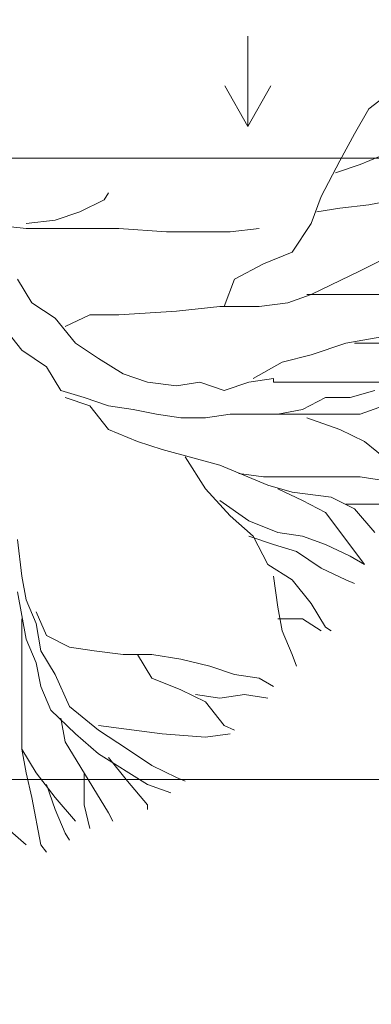
# Model space of a CAD drawing. Units: millimetres. Extents: x 595116 to 630915, y 909473 to 920225.
# Tile 18 of 134: x 629582 to 629596, y 919152 to 919190. Entities that reach past the tile are written whole.
import ezdxf

# ---------------------------------------------------------------- set-up
doc = ezdxf.new("R2010")
doc.units = ezdxf.units.MM
doc.layers.add('Dimension', color=3, linetype='Continuous', lineweight=18)
doc.layers.add('L-PLNT', color=85, linetype='Continuous', lineweight=13)
doc.styles.get("Standard").update_dxf_attribs({"font": 'arial.ttf'})
doc.dimstyles.new('ISO-25', dxfattribs={"dimtxt": 9, "dimasz": 6, "dimexe": 1.25, "dimexo": 0.625, "dimtad": 1, "dimlunit": 4, "dimtxsty": 'Standard', "dimcen": 2.5, "dimadec": 0, "dimazin": 0, "dimtfac": 1, "dimtmove": 0, "dimatfit": 3, "dimfxl": 1, "dimarcsym": 0})

# ---------------------------------------------------------------- blocks, each defined once
blk = doc.blocks.new('A$C143125F4')
for p, q in [((4.5624, 3.0105), (4.6554, 3.0821)), ((4.5077, 2.9164), (4.5624, 3.0105)), ((4.453, 2.8133), (4.5077, 2.9164)), ((4.5296, 2.7999), (4.639, 2.8447)), ((4.3819, 2.679), (4.453, 2.8133)), ((4.4366, 2.7686), (4.5296, 2.7999)), ((3.5613, 2.6655), (3.5777, 2.6924)), ((3.4683, 2.6207), (3.5613, 2.6655)), ((4.3436, 2.5759), (4.3819, 2.679)), ((4.453, 2.6342), (4.5624, 2.6476)), ((4.5624, 2.6476), (4.6554, 2.6655)), ((3.3753, 2.5894), (3.4683, 2.6207)), ((4.3655, 2.6207), (4.453, 2.6342)), ((3.0854, 2.5759), (3.2659, 2.558)), ((3.2659, 2.5759), (3.3753, 2.5894)), ((4.2725, 2.4684), (4.3436, 2.5759)), ((3.2659, 2.558), (3.616, 2.558)), ((3.616, 2.558), (3.7965, 2.5446)), ((3.7965, 2.5446), (4.0372, 2.5446)), ((4.0372, 2.5446), (4.1467, 2.558)), ((4.1631, 2.4236), (4.2725, 2.4684)), ((4.0537, 2.3654), (4.1631, 2.4236)), ((4.5296, 2.3967), (4.6171, 2.4415)), ((4.3436, 2.3071), (4.5296, 2.3967)), ((3.2878, 2.2758), (3.2331, 2.3654)), ((4.0154, 2.2623), (4.0537, 2.3654)), ((3.3753, 2.2175), (3.2878, 2.2758)), ((4.1467, 2.2623), (4.2561, 2.2758)), ((4.2561, 2.2758), (4.3436, 2.3071)), ((4.3272, 2.3071), (4.8906, 2.3071)), ((3.616, 2.231), (3.8348, 2.2444)), ((3.8348, 2.2444), (3.999, 2.2623)), ((3.999, 2.2623), (4.1467, 2.2623)), ((3.4519, 2.1235), (3.3753, 2.2175)), ((3.4136, 2.1862), (3.5066, 2.231)), ((3.5066, 2.231), (3.616, 2.231)), ((3.2495, 2.0966), (3.1784, 2.1862)), ((4.4749, 2.1235), (4.6554, 2.1548)), ((3.3425, 2.0339), (3.2495, 2.0966)), ((3.5394, 2.0652), (3.4519, 2.1235)), ((4.3436, 2.0787), (4.4749, 2.1235)), ((4.5077, 2.1235), (4.6171, 2.1235)), ((3.6324, 2.007), (3.5394, 2.0652)), ((4.1248, 1.9891), (4.2342, 2.0518)), ((4.2342, 2.0518), (4.3436, 2.0787)), ((3.3972, 1.9443), (3.3425, 2.0339)), ((3.7254, 1.9756), (3.6324, 2.007)), ((3.8348, 1.9622), (3.7254, 1.9756)), ((3.9224, 1.9756), (3.8348, 1.9622)), ((4.0154, 1.9443), (3.9224, 1.9756)), ((4.1084, 1.9756), (4.0154, 1.9443)), ((4.2014, 1.9891), (4.1084, 1.9756)), ((4.2014, 1.9756), (4.2014, 1.9891)), ((4.6718, 1.9756), (4.2014, 1.9756)), ((3.4847, 1.9174), (3.3972, 1.9443)), ((4.4913, 1.9174), (4.5843, 1.9443)), ((3.4136, 1.9174), (3.5066, 1.886)), ((3.5777, 1.886), (3.4847, 1.9174)), ((4.3108, 1.8726), (4.3983, 1.9174)), ((4.3983, 1.9174), (4.4913, 1.9174)), ((3.5066, 1.886), (3.5777, 1.7964)), ((3.6707, 1.8726), (3.5777, 1.886)), ((3.7583, 1.8547), (3.6707, 1.8726)), ((4.2178, 1.8547), (4.3108, 1.8726)), ((4.6171, 1.886), (4.5296, 1.8547)), ((3.8512, 1.8412), (3.7583, 1.8547)), ((3.9442, 1.8412), (3.8512, 1.8412)), ((4.0372, 1.8547), (3.9442, 1.8412)), ((4.1248, 1.8547), (4.0372, 1.8547)), ((4.5296, 1.8547), (4.1248, 1.8547)), ((4.3272, 1.8412), (4.453, 1.7964)), ((3.5777, 1.7964), (3.6871, 1.7516)), ((4.453, 1.7964), (4.546, 1.7516)), ((3.6871, 1.7516), (3.7801, 1.7203)), ((3.7801, 1.7203), (3.999, 1.662)), ((4.546, 1.7516), (4.639, 1.6755)), ((3.8677, 1.6934), (3.9442, 1.5724)), ((3.999, 1.662), (4.1795, 1.5859)), ((4.0701, 1.6307), (4.1631, 1.6172)), ((4.1631, 1.6172), (4.5296, 1.6172)), ((4.5296, 1.6172), (4.6171, 1.6038)), ((3.9442, 1.5724), (4.0372, 1.4694)), ((4.1795, 1.5859), (4.2725, 1.559)), ((4.2178, 1.5724), (4.3108, 1.5276)), ((4.2725, 1.559), (4.4202, 1.5411)), ((4.4202, 1.5411), (4.5077, 1.4963)), ((3.999, 1.5276), (4.1084, 1.4515)), ((4.3108, 1.5276), (4.3983, 1.4828)), ((4.4749, 1.5142), (4.6718, 1.5142)), ((4.5077, 1.4963), (4.5843, 1.4067)), ((4.0372, 1.4694), (4.1248, 1.3932)), ((4.3983, 1.4828), (4.4749, 1.3798)), ((4.1084, 1.4515), (4.2178, 1.4067)), ((3.2331, 1.3798), (3.2495, 1.2409)), ((4.1084, 1.3932), (4.2014, 1.3619)), ((4.1248, 1.3932), (4.1795, 1.2857)), ((4.2178, 1.4067), (4.3108, 1.3932)), ((4.3108, 1.3932), (4.3983, 1.3619)), ((4.4749, 1.3798), (4.546, 1.2857)), ((4.2014, 1.3619), (4.2889, 1.335)), ((4.3983, 1.3619), (4.4913, 1.3171)), ((4.2889, 1.335), (4.3819, 1.2723)), ((4.4913, 1.3171), (4.546, 1.2857)), ((4.1795, 1.2857), (4.2725, 1.2275)), ((4.3819, 1.2723), (4.4749, 1.2275)), ((3.2495, 1.2409), (3.2659, 1.1513)), ((4.2014, 1.2409), (4.2178, 1.1244)), ((4.2725, 1.2275), (4.3436, 1.1379)), ((4.4749, 1.2275), (4.5077, 1.214)), ((3.2659, 1.0035), (3.2331, 1.1827)), ((3.2659, 1.1513), (3.3042, 1.0617)), ((4.2178, 1.1244), (4.2342, 1.0348)), ((4.3436, 1.1379), (4.3983, 1.0483)), ((3.3042, 1.1065), (3.3425, 1.0169)), ((3.2495, 1.0796), (3.2495, 0.5869)), ((3.3042, 1.0617), (3.3206, 0.9587)), ((4.2178, 1.0796), (4.3108, 1.0796)), ((4.3108, 1.0796), (4.3819, 1.0348)), ((4.3983, 1.0483), (4.4202, 1.0348)), ((3.3425, 1.0169), (3.43, 0.9721)), ((4.2342, 1.0348), (4.2725, 0.9452)), ((3.3042, 0.9139), (3.2659, 1.0035)), ((3.43, 0.9721), (3.523, 0.9587)), ((3.3206, 0.9587), (3.3753, 0.8691)), ((3.523, 0.9587), (3.6324, 0.9452)), ((3.6324, 0.9452), (3.7418, 0.9452)), ((3.6871, 0.9452), (3.7418, 0.8557)), ((3.7418, 0.9452), (3.8512, 0.9273)), ((4.2725, 0.9452), (4.2889, 0.9005)), ((3.3206, 0.8243), (3.3042, 0.9139)), ((3.8512, 0.9273), (3.9607, 0.9005)), ((3.9607, 0.9005), (4.0537, 0.8691)), ((3.3753, 0.8691), (3.43, 0.7481)), ((4.0537, 0.8691), (4.1467, 0.8557)), ((3.3589, 0.7347), (3.3206, 0.8243)), ((3.7418, 0.8557), (3.8512, 0.8109)), ((4.1467, 0.8557), (4.2014, 0.8243)), ((3.8512, 0.8109), (3.9442, 0.7661)), ((3.906, 0.7929), (3.999, 0.7795)), ((3.999, 0.7795), (4.092, 0.7929)), ((4.092, 0.7929), (4.1795, 0.7795)), ((3.43, 0.7481), (3.5394, 0.6585)), ((3.9442, 0.7661), (4.0154, 0.6765)), ((3.4519, 0.6451), (3.3589, 0.7347)), ((3.3972, 0.7033), (3.4136, 0.6137)), ((3.5394, 0.6765), (3.7801, 0.6451)), ((4.0154, 0.6765), (4.0537, 0.6585)), ((3.5394, 0.5689), (3.4519, 0.6451)), ((3.5394, 0.6585), (3.6488, 0.5869)), ((3.7801, 0.6451), (3.9442, 0.6317)), ((3.9442, 0.6317), (4.0372, 0.6451)), ((3.4136, 0.6137), (3.5777, 0.3449)), ((3.2495, 0.5869), (3.3042, 0.4973)), ((3.2495, 0.5869), (3.2659, 0.4973)), ((3.7254, 0.4525), (3.5394, 0.5689)), ((3.6488, 0.5869), (3.7418, 0.5241)), ((3.5777, 0.5555), (3.6488, 0.4659)), ((3.7418, 0.5241), (3.8348, 0.4793)), ((3.2659, 0.4973), (3.2878, 0.4032)), ((3.3042, 0.4973), (3.3753, 0.4032)), ((3.4847, 0.4973), (3.4847, 0.3763)), ((3.3425, 0.4525), (3.3753, 0.3584)), ((3.6488, 0.4659), (3.7254, 0.3763)), ((3.813, 0.4211), (3.7254, 0.4525)), ((3.8348, 0.4793), (3.8677, 0.4659)), ((3.2878, 0.4032), (3.3206, 0.224)), ((3.3753, 0.4032), (3.4519, 0.3136)), ((3.4847, 0.3763), (3.5066, 0.2867)), ((3.7254, 0.3763), (3.7254, 0.3584)), ((3.3753, 0.3584), (3.4136, 0.2688)), ((3.5777, 0.3449), (3.5941, 0.3136)), ((3.1948, 0.2867), (3.2659, 0.224)), ((3.4136, 0.2688), (3.43, 0.2419)), ((3.3206, 0.224), (3.3425, 0.1971))]:
    blk.add_line(p, q)
blk = doc.blocks.new('LAWN-GRASS-TUFT')
blk.add_line((0.892, 3.485), (0.892, 0))
blk.add_lwpolyline([(0, 1.577), (0.892, 0), (1.785, 1.577)])
blk = doc.blocks.new('*D216')
at = {"layer": 'Defpoints', "color": 0, "transparency": 16777216}
for p in [(629505.041, 919411.828), (629743.541, 919411.928), (629743.541, 918832.378)]:
    blk.add_point(p, dxfattribs=at)
at = {"layer": 'Dimension', "color": 0, "lineweight": -2, "transparency": 16777216}
for p, q in [((629505.041, 919411.203), (629505.041, 918831.128)), ((629743.541, 919411.303), (629743.541, 918831.128)), ((629511.041, 918832.378), (629737.541, 918832.378))]:
    blk.add_line(p, q, dxfattribs=at)
at = {"layer": 'Dimension', "color": 0, "transparency": 16777216}
for points in [[(629511.041, 918833.378), (629511.041, 918831.378), (629505.041, 918832.378)], [(629737.541, 918833.378), (629737.541, 918831.378), (629743.541, 918832.378)]]:
    blk.add_solid(points, dxfattribs=at)
at = {"layer": 'Dimension', "color": 0, "transparency": 16777216, "insert": (629624.291, 918837.656), "char_height": 9, "attachment_point": 5}
blk.add_mtext('19\'-10 1/2"', dxfattribs=at)

msp = doc.modelspace()

# ---------------------------------------------------------------- linework, layer by layer
at = {"layer": 'L-PLNT'}
for p, q in [((629535.274, 919184.917), (629800.951, 919184.917)), ((629511.274, 919160.917), (629824.951, 919160.917))]:
    msp.add_line(p, q, dxfattribs=at)

# ---------------------------------------------------------------- block references
at = {"layer": 'L-PLNT', "xscale": 10.20167662382051, "yscale": 10.20167662382051, "zscale": 10.20167662382051}
msp.add_blockref('A$C143125F4', (629549.214, 919156.111), dxfattribs=at)
at = {"layer": 'L-PLNT'}
msp.add_blockref('LAWN-GRASS-TUFT', (629590.192, 919186.14), dxfattribs=at)

# ---------------------------------------------------------------- dimensions: what is measured, and where the dimension line sits
at = {"layer": 'Dimension'}
dim = msp.add_linear_dim(base=(629743.541, 918832.378), p1=(629505.041, 919411.828), p2=(629743.541, 919411.928), dimstyle='ISO-25', override={"dimdec": 1, "dimlfac": 1, "dimrnd": 0, "dimzin": 1, "dimdsep": 46, "dimlunit": 4, "dimfrac": 2}, dxfattribs=at)
dim.commit()
dim.dimension.update_dxf_attribs({"geometry": '*D216', "text_midpoint": (629624.291, 918837.656)})

doc.saveas('drawing.dxf')
